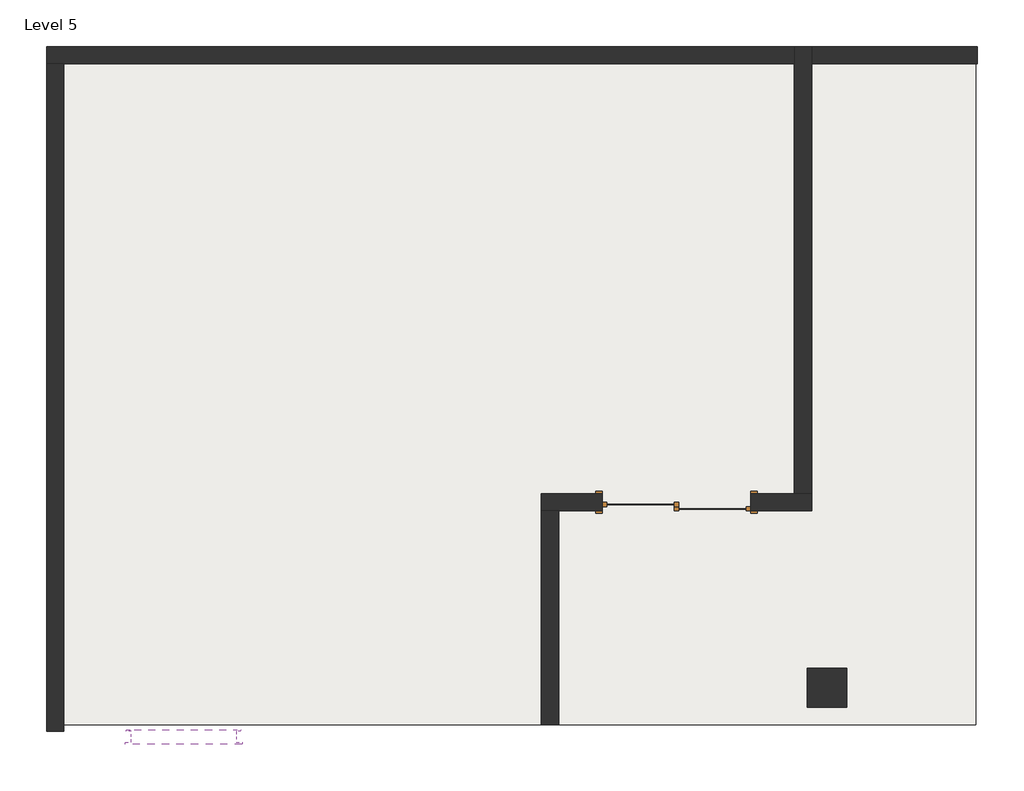
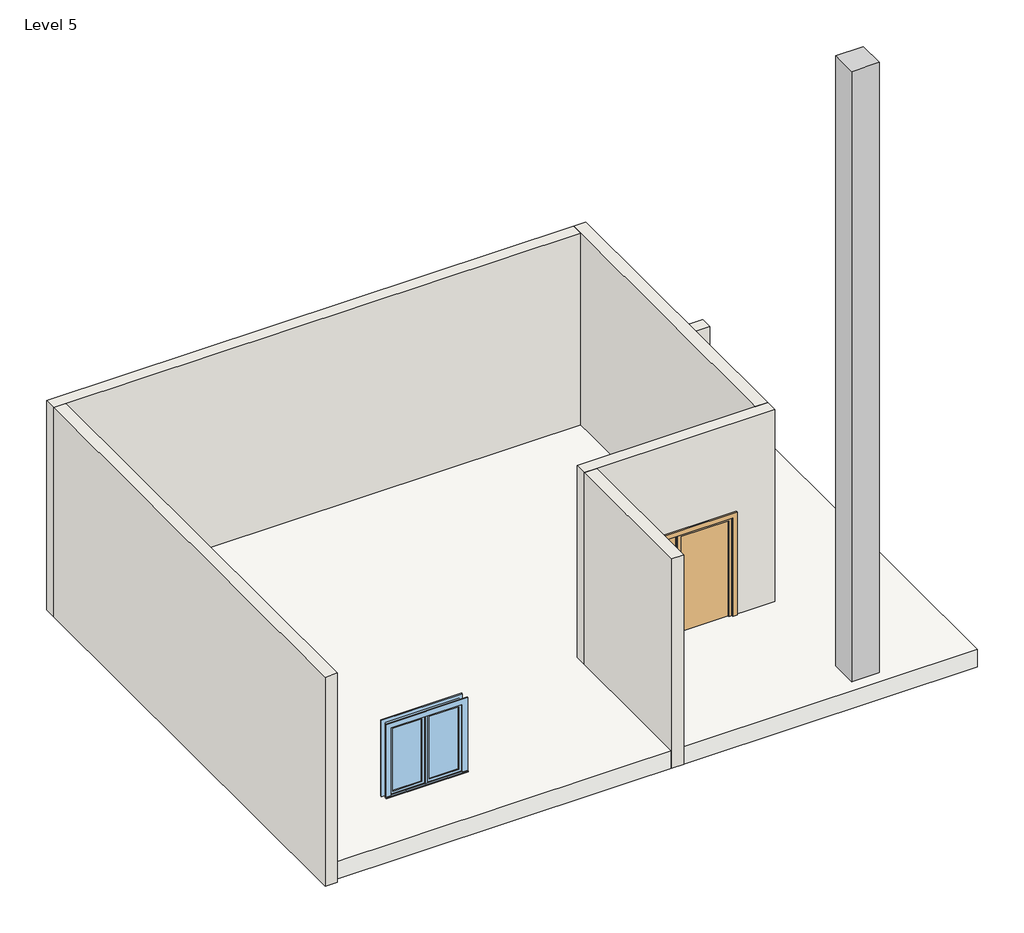
# One storey: 6 walls, 1 column, 1 door, 1 roof, 1 window.
"""IFC4 building model written with IfcOpenShell, lengths in millimetres."""

from ifc_helpers import new_model, si_unit, frame, origin, place, context, project, spatial, polyline, outline, extrude, faceted_brep, transform, mapped, element, save
from components import door_076b30e0, window_40d2abec

model = new_model("IFC4")

# Units and contexts
model_context = context("Model", 3, world=origin())
ifc_project = project(units=[si_unit("LENGTHUNIT", "METRE", prefix="MILLI")], contexts=[model_context])

# Site, building, storey
site = spatial("IfcSite", under=ifc_project)
building = spatial("IfcBuilding", under=site)
storey = spatial("IfcBuildingStorey", under=building, Name="Level 5", Elevation=14630.4)

# Column
placement = place(None, origin())
element("IfcColumn", 1, ObjectType="Rectangular Column : 18\" x 18\"", at=placement, inside=storey, context=model_context, shape_type="Brep", body=[
    faceted_brep([(-4893.9304753, 3719.2297737, 25603.2), (-5351.1304753, 3719.2297737, 25603.2), (-5351.1304753, 3262.0297737, 25603.2), (-5249.5304753, 3262.0297737, 25603.2), (-5097.1304753, 3262.0297737, 25603.2), (-4944.7304753, 3262.0297737, 25603.2), (-4893.9304753, 3262.0297737, 25603.2), (-4893.9304753, 3719.2297737, 14935.2), (-4893.9304753, 3262.0297737, 14935.2), (-5351.1304753, 3262.0297737, 14935.2), (-5351.1304753, 3719.2297737, 14935.2), (-4893.9304753, 3262.0297737, 22250.4)], [[[0, 1, 2, 3, 4, 5, 6]], [[7, 8, 9, 10]], [[1, 0, 7, 10]], [[2, 1, 10, 9]], [[6, 5, 4, 3, 2, 9, 8, 11]], [[0, 6, 11, 8, 7]]]),
])

# Door
door_shape = door_076b30e0(model_context)
element("IfcDoor", 2, ObjectType="Door-Double-Sliding : 68\" x 80\"", at=placement, inside=storey, context=model_context, shape_type="MappedRepresentation", body=[
    mapped(door_shape, transform((-6875.1304753, 5777.4732783, 14630.4), x_axis=(-1.0, 0.0, 0.0), y_axis=(0.0, -1.0, 0.0), z_axis=(0.0, 0.0, 1.0))),
])

# Roof
element("IfcRoof", 3, ObjectType="Generic - 12\"", at=placement, inside=storey, context=model_context, shape_type="SweptSolid", body=[
    extrude(outline(polyline([(-14209.7864811, 10932.8297737), (-3389.3864811, 10932.8297737), (-3389.3864811, 3058.8297737), (-14209.7864811, 3058.8297737), (-14209.7864811, 10932.8297737)])), frame((0.0, 0.0, 14630.4), z_axis=(0.0, 0.0, 1.0), x_axis=(1.0, 0.0, 0.0)), (0.0, 0.0, 1.0), 304.8),
])

# Walls
element("IfcWall", 4, ObjectType="Generic - 8\"", at=placement, inside=storey, context=model_context, shape_type="Brep", body=[
    faceted_brep([(-7738.7304753, 5752.0732783, 16662.4), (-7738.7304753, 5752.0732783, 14630.4), (-8449.9304753, 5752.0732783, 14630.4), (-8449.9304753, 5752.0732783, 18288.0), (-5503.5304753, 5752.0732783, 18288.0), (-5300.3304753, 5752.0732783, 18288.0), (-5300.3304753, 5752.0732783, 14630.4), (-5503.5304753, 5752.0732783, 14630.4), (-6011.5304753, 5752.0732783, 14630.4), (-6011.5304753, 5752.0732783, 16662.4), (-8449.9304753, 5548.8732783, 14630.4), (-8246.7304753, 5548.8732783, 14630.4), (-7738.7304753, 5548.8732783, 14630.4), (-7738.7304753, 5548.8732783, 16662.4), (-6011.5304753, 5548.8732783, 16662.4), (-6011.5304753, 5548.8732783, 14630.4), (-5300.3304753, 5548.8732783, 14630.4), (-5300.3304753, 5548.8732783, 18288.0), (-8246.7304753, 5548.8732783, 18288.0), (-8449.9304753, 5548.8732783, 18288.0)], [[[0, 1, 2, 3, 4, 5, 6, 7, 8, 9]], [[10, 11, 12, 13, 14, 15, 16, 17, 18, 19]], [[2, 1, 12, 11, 10]], [[8, 7, 6, 16, 15]], [[5, 4, 3, 19, 18, 17]], [[3, 2, 10, 19]], [[6, 5, 17, 16]], [[15, 14, 9, 8]], [[13, 12, 1, 0]], [[14, 13, 0, 9]]]),
])
element("IfcWall", 5, ObjectType="Generic - 8\"", at=placement, inside=storey, context=model_context, shape_type="SweptSolid", body=[
    extrude(outline(polyline([(-8449.9304753, 3058.8297737), (-8449.9304753, 5548.8732783), (-8246.7304753, 5548.8732783), (-8246.7304753, 3058.8297737), (-8449.9304753, 3058.8297737)])), frame((0.0, 0.0, 14630.4), z_axis=(0.0, 0.0, 1.0), x_axis=(1.0, 0.0, 0.0)), (0.0, 0.0, 1.0), 3657.6),
])
element("IfcWall", 6, ObjectType="Generic - 8\"", at=placement, inside=storey, context=model_context, shape_type="Brep", body=[
    faceted_brep([(-5300.3304753, 5752.0732783, 14630.4), (-5300.3304753, 10958.2297737, 14630.4), (-5300.3304753, 10958.2297737, 14917.2125244), (-5300.3304753, 10958.2297737, 15906.0392493), (-5300.3304753, 10958.2297737, 18288.0), (-5300.3304753, 5752.0732783, 18288.0), (-5503.5304753, 5752.0732783, 14630.4), (-5503.5304753, 5752.0732783, 18288.0), (-5503.5304753, 10755.0297737, 18288.0), (-5503.5304753, 10958.2297737, 18288.0), (-5503.5304753, 10958.2297737, 14630.4), (-5503.5304753, 10755.0297737, 14630.4)], [[[0, 1, 2, 3, 4, 5]], [[6, 7, 8, 9, 10, 11]], [[1, 0, 6, 11, 10]], [[5, 4, 9, 8, 7]], [[0, 5, 7, 6]], [[1, 10, 9, 4, 3, 2]]]),
])
element("IfcWall", 7, ObjectType="Generic - 8\"", at=placement, inside=storey, context=model_context, shape_type="Brep", body=[
    faceted_brep([(-5503.5304753, 10958.2297737, 18288.0), (-5503.5304753, 10958.2297737, 14630.4), (-14212.6992777, 10958.2297737, 14630.4), (-14212.6992777, 10958.2297737, 18288.0), (-5503.5304753, 10755.0297737, 14630.4), (-5503.5304753, 10755.0297737, 18288.0), (-14009.4992777, 10755.0297737, 18288.0), (-14212.6992777, 10755.0297737, 18288.0), (-14212.6992777, 10755.0297737, 14630.4), (-14009.4992777, 10755.0297737, 14630.4)], [[[0, 1, 2, 3]], [[4, 5, 6, 7, 8, 9]], [[2, 1, 4, 9, 8]], [[0, 3, 7, 6, 5]], [[3, 2, 8, 7]], [[0, 5, 4, 1]]]),
])
element("IfcWall", 8, ObjectType="Generic - 8\"", at=placement, inside=storey, context=model_context, shape_type="SweptSolid", body=[
    extrude(outline(polyline([(-14212.6992777, 2982.6297737), (-14212.6992777, 10755.0297737), (-14009.4992777, 10755.0297737), (-14009.4992777, 2982.6297737), (-14212.6992777, 2982.6297737)])), frame((0.0, 0.0, 14630.4), z_axis=(0.0, 0.0, 1.0), x_axis=(1.0, 0.0, 0.0)), (0.0, 0.0, 1.0), 3657.6),
])
element("IfcWall", 9, ObjectType="Generic - 8\"", at=placement, inside=storey, context=model_context, shape_type="SweptSolid", body=[
    extrude(outline(polyline([(-3369.9304753, 10755.0297737), (-5300.3304753, 10755.0297737), (-5300.3304753, 10958.2297737), (-3369.9304753, 10958.2297737), (-3369.9304753, 10755.0297737)])), frame((0.0, 0.0, 14917.2125244), z_axis=(0.0, 0.0, 1.0), x_axis=(1.0, 0.0, 0.0)), (0.0, 0.0, 1.0), 988.8267249),
])

# Window
window_shape = window_40d2abec(model_context)
element("IfcWindow", 10, ObjectType="Casement Dbl with Trim.0001 : 48\" x 48\"", at=placement, inside=storey, context=model_context, shape_type="MappedRepresentation", body=[
    mapped(window_shape, transform((-12615.5304753, 2938.1797737, 15016.504066), x_axis=(-1.0, 0.0, 0.0), y_axis=(0.0, -1.0, 0.0), z_axis=(0.0, 0.0, 1.0))),
])

save(model, "model.ifc")

# Revit data of these elements
# Type "Rectangular Column : 18\" x 18\""
#   Assembly Code = "B1010200"
#   Depth = 1' - 6"
#   Offset Base = 0' - 0"
#   Offset Top = 0' - 0"
#   Width = 1' - 6"
#   Material = none
# Type "Door-Double-Sliding : 68\" x 80\""
#   Type Mark = "8"
#   Construction Type Id = "opn-d45"
#   Assembly Code = "C1020"
#   Analytic Construction = "Wood frame, double glass door "
#   Thickness = 0' - 2"
#   Thermal Resistance (R) = 1.8150 (h·ft²·°F)/BTU
#   Heat Transfer Coefficient (U) = 0.5510 BTU/(h·ft²·°F)
#   Height = 6' - 8"
#   Rail Width = 0' - 2"
#   Stiles = 0' - 2"
#   Trim Projection Ext = 0' - 1"
#   Trim Projection Int = 0' - 1"
#   Trim Width = 0' - 3"
#   Width = 5' - 8"
#   Define Thermal Properties by = 1
#   Glazing = Glass
#   Panel Material = Wood - Birch - Solid Stained Light Low Gloss
#   Trim Material = Paint - Sienna
#   Visual Light Transmittance = 0
#   Solar Heat Gain Coefficient = 0
#   Function = (empty or 0)
#   Wall Closure = (empty or 0)
# Type "Generic - 12\""
#   Assembly Code = "B1020"
#   Layers, outside or top first: 1' - 0" no material (function 1)
# Type "Generic - 8\""
#   Assembly Code = "B2010"
#   Layers, outside or top first: 0' - 8" no material (function 1)
# Type "Casement Dbl with Trim.0001 : 48\" x 48\""
#   Type Mark = "10"
#   Construction Type Id = "GSP4R"
#   Assembly Code = "B2020100"
#   Analytic Construction = "1/8 in Pilkington single glazing"
#   Visual Light Transmittance = 0.9
#   Solar Heat Gain Coefficient = 0.78
#   Heat Transfer Coefficient (U) = 0.6496 BTU/(h·ft²·°F)
#   Height = 4' - 0"
#   Default Sill Height = 3' - 0"
#   Trim Projection - Ext. = 0' - 0 1/2"
#   Trim Projection - Int. = 0' - 0 3/4"
#   Trim Width - Exterior = 0' - 3 1/2"
#   Trim Width - Interior = 0' - 3 1/2"
#   Width = 4' - 0"
#   Window Inset = 0' - 0 3/4"
#   Define Thermal Properties by = 1
#   Glass Pane Material = Glass
#   Sash Material = Sash
#   Trim Exterior Material = Trim
#   Trim Interior Material = Trim
#   Wall Closure = (empty or 0)
# Element 1 (IfcColumn, "Rectangular Column : 18\" x 18\"")
#   Phase Created = New Construction
#   Materials on its faces: "Default Wall"
# Element 2 (IfcDoor, "Door-Double-Sliding : 68\" x 80\"")
#   Phase Created = New Construction
#   Materials on its faces: "Paint - Sienna", "Wood - Birch - Solid Stained Light Low Gloss", "Glass"
# Element 3 (IfcRoof, "Generic - 12\"")
#   built-in parameter 1001705 = 49 (stored number, unit not read)
#   built-in parameter 1001710 = 33615
#   Phase Created = New Construction
#   Materials on its faces: "Default Roof"
# Elements 4, 5, 6, 7, 8 (IfcWall, "Generic - 8\"")
#   Top Offset = 0' - 0"
#   Base Offset = 0' - 0"
#   Unconnected Height = 12' - 0"
#   wall height = 12' - 0"
#   Phase Created = New Construction
#   Base Constraint = Level 5
#   Materials on its faces: "Default Wall"
# Element 9 (IfcWall, "Generic - 8\"")
#   built-in parameter 1001111 = 0' - 11.29183"
#   Top Offset = 0' - 0"
#   Base Offset = 0' - 11.29183"
#   Unconnected Height = 3' - 2.93019"
#   wall height = 3' - 2.93019"
#   Phase Created = New Construction
#   Base Constraint = Level 5
#   Materials on its faces: "Default Wall"
# Element 10 (IfcWindow, "Casement Dbl with Trim.0001 : 48\" x 48\"")
#   Mark = "5"
#   Phase Created = New Construction
#   Materials on its faces: "Sash", "Trim", "Glass"
# Materials
#   "Glass": class "Glass", colour RGB 0 128 192, transparency 0.75, Description = "Soda Lime Glass", Cost = 0
#   "Wood - Birch - Solid Stained Light Low Gloss": class "Wood", colour RGB 210 159 95, transparency 0, Cost = 0
#   "Paint - Sienna": colour RGB 118 70 51, transparency 0, Cost = 0
#   "Sash": class "Wood", colour RGB 224 178 126, transparency 0
#   "Trim": class "Wood", colour RGB 224 178 126, transparency 0
#   "Default Wall": colour RGB 128 128 128, transparency 0
#   "Default Roof": colour RGB 88 101 114, transparency 0
